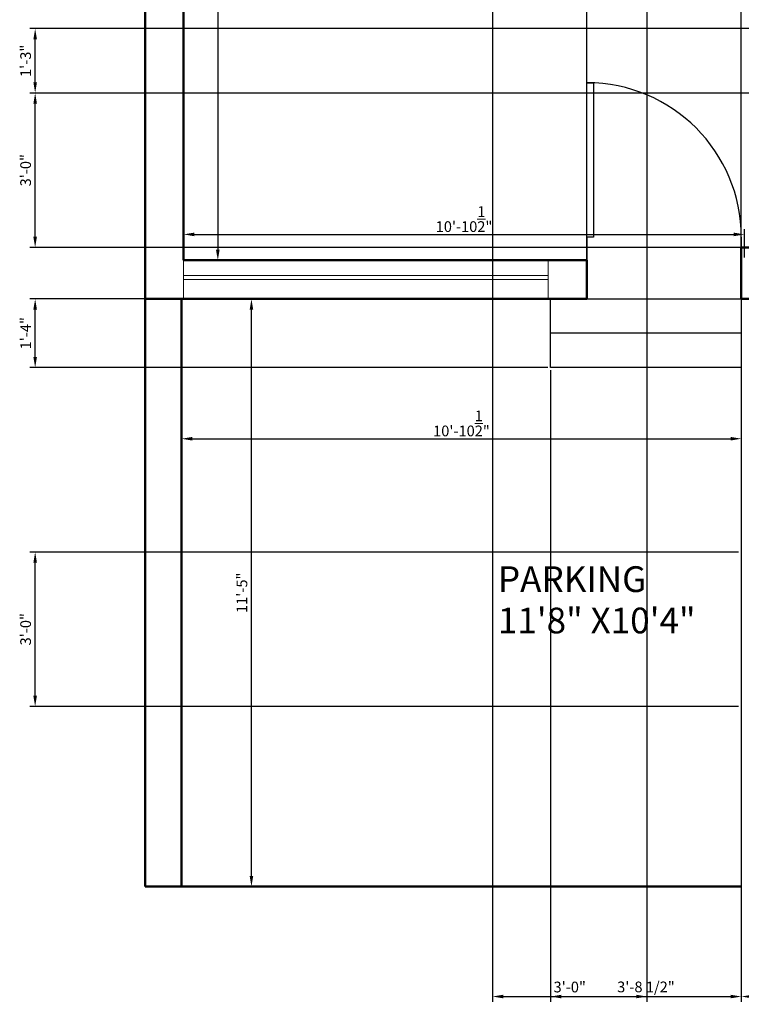
# Model space of a CAD drawing. Units: inches. Extents: x 2385 to 2740, y 1752 to 2305.
# Tile 1 of 15: x 2385 to 2553, y 1752 to 1981. Entities that reach past the tile are written whole.
import ezdxf

# ---------------------------------------------------------------- set-up
doc = ezdxf.new("R2010")
doc.units = ezdxf.units.IN
for name, color, linetype, lineweight in [('A-ANNO-DIMS', 2, 'Continuous', 18), ('A-AREA-IDEN', 7, 'Continuous', 25), ('A-DOOR', 4, 'Continuous', 25), ('A-FLOR-STRS', 7, 'Continuous', 25), ('A-GLAZ', 4, 'Continuous', 18), ('A-WALL', 7, 'Continuous', 50)]:
    doc.layers.add(name, color=color, linetype=linetype, lineweight=lineweight)
doc.styles.get("Standard").update_dxf_attribs({"font": 'arial.ttf'})
doc.dimstyles.new('Copy of ISO-25', dxfattribs={"dimtxt": 2.5, "dimasz": 2.5, "dimexe": 1.25, "dimexo": 0.625, "dimtad": 1, "dimdec": 1, "dimlunit": 4, "dimtxsty": 'Standard', "dimcen": 2.5, "dimadec": 0, "dimazin": 0, "dimtfac": 1, "dimtdec": 1, "dimtmove": 0, "dimatfit": 3, "dimfxl": 1, "dimarcsym": 0})

# ---------------------------------------------------------------- blocks, each defined once
blk = doc.blocks.new('*D12')
at = {"layer": 'A-ANNO-DIMS', "color": 0, "lineweight": -2, "transparency": 16777216}
for p, q in [((2423.87, 2140.97), (2432.46, 2140.97)), ((2431.21, 2138.47), (2431.21, 1927.47)), ((2423.87, 1924.97), (2432.46, 1924.97))]:
    blk.add_line(p, q, dxfattribs=at)
at = {"layer": 'A-ANNO-DIMS', "color": 0, "transparency": 16777216}
for points in [[(2430.79, 2138.47), (2431.63, 2138.47), (2431.21, 2140.97)], [(2430.79, 1927.47), (2431.63, 1927.47), (2431.21, 1924.97)]]:
    blk.add_solid(points, dxfattribs=at)
at = {"layer": 'Defpoints', "color": 0, "transparency": 16777216}
for p in [(2423.25, 2140.97), (2423.25, 1924.97), (2431.21, 1924.97)]:
    blk.add_point(p, dxfattribs=at)
at = {"layer": 'A-ANNO-DIMS', "color": 0, "transparency": 16777216, "insert": (2429.31, 2032.97), "char_height": 2.5, "attachment_point": 5, "rotation": 90}
blk.add_mtext("18'", dxfattribs=at)
blk = doc.blocks.new('*D13')
at = {"layer": 'A-ANNO-DIMS', "color": 0, "lineweight": -2, "transparency": 16777216}
for p, q in [((2423.25, 1925.59), (2423.25, 1932.26)), ((2425.75, 1931.01), (2551.46, 1931.01)), ((2553.96, 1925.59), (2553.96, 1932.26))]:
    blk.add_line(p, q, dxfattribs=at)
at = {"layer": 'A-ANNO-DIMS', "color": 0, "transparency": 16777216}
for points in [[(2425.75, 1931.43), (2425.75, 1930.59), (2423.25, 1931.01)], [(2551.46, 1931.43), (2551.46, 1930.59), (2553.96, 1931.01)]]:
    blk.add_solid(points, dxfattribs=at)
at = {"layer": 'Defpoints', "color": 0, "transparency": 16777216}
for p in [(2553.96, 1931.01), (2423.25, 1924.97), (2553.96, 1924.97)]:
    blk.add_point(p, dxfattribs=at)
at = {"layer": 'A-ANNO-DIMS', "color": 0, "transparency": 16777216, "insert": (2488.61, 1934.58), "char_height": 2.5, "attachment_point": 5}
blk.add_mtext('10\'-10{\\H1x;\\S1/2;}"', dxfattribs=at)
blk = doc.blocks.new('*D20')
at = {"layer": 'A-ANNO-DIMS', "color": 0, "lineweight": -2, "transparency": 16777216}
for p, q in [((2423.4, 1915.97), (2440.3, 1915.97)), ((2439.05, 1781.47), (2439.05, 1913.47)), ((2423.4, 1778.97), (2440.3, 1778.97))]:
    blk.add_line(p, q, dxfattribs=at)
at = {"layer": 'A-ANNO-DIMS', "color": 0, "transparency": 16777216}
for points in [[(2438.64, 1913.47), (2439.47, 1913.47), (2439.05, 1915.97)], [(2438.64, 1781.47), (2439.47, 1781.47), (2439.05, 1778.97)]]:
    blk.add_solid(points, dxfattribs=at)
at = {"layer": 'Defpoints', "color": 0, "transparency": 16777216}
for p in [(2422.77, 1915.97), (2439.05, 1915.97), (2422.77, 1778.97)]:
    blk.add_point(p, dxfattribs=at)
at = {"layer": 'A-ANNO-DIMS', "color": 0, "transparency": 16777216, "insert": (2437.15, 1847.47), "char_height": 2.5, "attachment_point": 5, "rotation": 90}
blk.add_mtext('11\'-5"', dxfattribs=at)
blk = doc.blocks.new('*D21')
at = {"layer": 'A-ANNO-DIMS', "color": 0, "lineweight": -2, "transparency": 16777216}
for p, q in [((2422.77, 1915.34), (2422.77, 1882.13)), ((2553.25, 1915.34), (2553.25, 1882.13)), ((2425.27, 1883.38), (2550.75, 1883.38))]:
    blk.add_line(p, q, dxfattribs=at)
at = {"layer": 'A-ANNO-DIMS', "color": 0, "transparency": 16777216}
for points in [[(2425.27, 1883.8), (2425.27, 1882.96), (2422.77, 1883.38)], [(2550.75, 1883.8), (2550.75, 1882.96), (2553.25, 1883.38)]]:
    blk.add_solid(points, dxfattribs=at)
at = {"layer": 'Defpoints', "color": 0, "transparency": 16777216}
for p in [(2422.77, 1915.97), (2553.25, 1915.97), (2553.25, 1883.38)]:
    blk.add_point(p, dxfattribs=at)
at = {"layer": 'A-ANNO-DIMS', "color": 0, "transparency": 16777216, "insert": (2488.01, 1886.95), "char_height": 2.5, "attachment_point": 5}
blk.add_mtext('10\'-10{\\H1x;\\S1/2;}"', dxfattribs=at)
blk = doc.blocks.new('*U23')
for p, q in [((0, 0), (0, -6)), ((40, 0), (40, -6))]:
    blk.add_line(p, q)
blk.add_lwpolyline([(0, 0), (0, 40), (1.75, 40), (1.75, 0)], close=True)
blk.add_arc((0, 0), 40, 0, 90)
blk = doc.blocks.new('*D34')
at = {"layer": 'A-ANNO-DIMS', "color": 0, "lineweight": -2, "transparency": 16777216}
for p, q in [((2553.25, 1820.34), (2553.25, 1752.1)), ((2651.25, 1820.34), (2651.25, 1752.1)), ((2555.75, 1753.35), (2648.75, 1753.35))]:
    blk.add_line(p, q, dxfattribs=at)
at = {"layer": 'A-ANNO-DIMS', "color": 0, "transparency": 16777216}
for points in [[(2555.75, 1753.77), (2555.75, 1752.94), (2553.25, 1753.35)], [(2648.75, 1753.77), (2648.75, 1752.94), (2651.25, 1753.35)]]:
    blk.add_solid(points, dxfattribs=at)
at = {"layer": 'Defpoints', "color": 0, "transparency": 16777216}
for p in [(2553.25, 1820.97), (2651.25, 1820.97), (2651.25, 1753.35)]:
    blk.add_point(p, dxfattribs=at)
at = {"layer": 'A-ANNO-DIMS', "color": 0, "transparency": 16777216, "insert": (2602.25, 1755.25), "char_height": 2.5, "attachment_point": 5}
blk.add_mtext('8\'-2"', dxfattribs=at)
blk = doc.blocks.new('*D35')
at = {"layer": 'A-ANNO-DIMS', "color": 0, "lineweight": -2, "transparency": 16777216}
for p, q in [((2552.62, 1856.97), (2387.38, 1856.97)), ((2388.63, 1823.47), (2388.63, 1854.47)), ((2552.62, 1820.97), (2387.38, 1820.97))]:
    blk.add_line(p, q, dxfattribs=at)
at = {"layer": 'A-ANNO-DIMS', "color": 0, "transparency": 16777216}
for points in [[(2388.21, 1854.47), (2389.05, 1854.47), (2388.63, 1856.97)], [(2388.21, 1823.47), (2389.05, 1823.47), (2388.63, 1820.97)]]:
    blk.add_solid(points, dxfattribs=at)
at = {"layer": 'Defpoints', "color": 0, "transparency": 16777216}
for p in [(2388.63, 1856.97), (2553.25, 1856.97), (2553.25, 1820.97)]:
    blk.add_point(p, dxfattribs=at)
at = {"layer": 'A-ANNO-DIMS', "color": 0, "transparency": 16777216, "insert": (2386.73, 1838.97), "char_height": 2.5, "attachment_point": 5, "rotation": 90}
blk.add_mtext('3\'-0"', dxfattribs=at)
blk = doc.blocks.new('*D37')
at = {"layer": 'A-ANNO-DIMS', "color": 0, "lineweight": -2, "transparency": 16777216}
for p, q in [((2495.25, 2140.34), (2495.25, 1752.1)), ((2531.25, 2140.34), (2531.25, 1752.1)), ((2497.75, 1753.35), (2528.75, 1753.35))]:
    blk.add_line(p, q, dxfattribs=at)
at = {"layer": 'A-ANNO-DIMS', "color": 0, "transparency": 16777216}
for points in [[(2497.75, 1753.77), (2497.75, 1752.94), (2495.25, 1753.35)], [(2528.75, 1753.77), (2528.75, 1752.94), (2531.25, 1753.35)]]:
    blk.add_solid(points, dxfattribs=at)
at = {"layer": 'Defpoints', "color": 0, "transparency": 16777216}
for p in [(2495.25, 2140.97), (2531.25, 2140.97), (2531.25, 1753.35)]:
    blk.add_point(p, dxfattribs=at)
at = {"layer": 'A-ANNO-DIMS', "color": 0, "transparency": 16777216, "insert": (2513.25, 1755.25), "char_height": 2.5, "attachment_point": 5}
blk.add_mtext('3\'-0"', dxfattribs=at)
blk = doc.blocks.new('*D41')
at = {"layer": 'A-ANNO-DIMS', "color": 0, "lineweight": -2, "transparency": 16777216}
for p, q in [((2558.62, 1978.97), (2387.38, 1978.97)), ((2388.63, 1966.47), (2388.63, 1976.47)), ((2558.62, 1963.97), (2387.38, 1963.97))]:
    blk.add_line(p, q, dxfattribs=at)
at = {"layer": 'A-ANNO-DIMS', "color": 0, "transparency": 16777216}
for points in [[(2388.21, 1976.47), (2389.05, 1976.47), (2388.63, 1978.97)], [(2388.21, 1966.47), (2389.05, 1966.47), (2388.63, 1963.97)]]:
    blk.add_solid(points, dxfattribs=at)
at = {"layer": 'Defpoints', "color": 0, "transparency": 16777216}
for p in [(2388.63, 1978.97), (2559.25, 1978.97), (2559.25, 1963.97)]:
    blk.add_point(p, dxfattribs=at)
at = {"layer": 'A-ANNO-DIMS', "color": 0, "transparency": 16777216, "insert": (2386.73, 1971.47), "char_height": 2.5, "attachment_point": 5, "rotation": 90}
blk.add_mtext('1\'-3"', dxfattribs=at)
blk = doc.blocks.new('*D42')
at = {"layer": 'A-ANNO-DIMS', "color": 0, "lineweight": -2, "transparency": 16777216}
for p, q in [((2558.62, 1963.97), (2387.38, 1963.97)), ((2388.63, 1930.47), (2388.63, 1961.47)), ((2558.62, 1927.97), (2387.38, 1927.97))]:
    blk.add_line(p, q, dxfattribs=at)
at = {"layer": 'A-ANNO-DIMS', "color": 0, "transparency": 16777216}
for points in [[(2388.21, 1961.47), (2389.05, 1961.47), (2388.63, 1963.97)], [(2388.21, 1930.47), (2389.05, 1930.47), (2388.63, 1927.97)]]:
    blk.add_solid(points, dxfattribs=at)
at = {"layer": 'Defpoints', "color": 0, "transparency": 16777216}
for p in [(2388.63, 1963.97), (2559.25, 1963.97), (2559.25, 1927.97)]:
    blk.add_point(p, dxfattribs=at)
at = {"layer": 'A-ANNO-DIMS', "color": 0, "transparency": 16777216, "insert": (2386.73, 1945.97), "char_height": 2.5, "attachment_point": 5, "rotation": 90}
blk.add_mtext('3\'-0"', dxfattribs=at)
blk = doc.blocks.new('*D46')
at = {"layer": 'A-ANNO-DIMS', "color": 0, "lineweight": -2, "transparency": 16777216}
for p, q in [((2508.79, 1899.34), (2508.79, 1752.1)), ((2553.25, 1899.34), (2553.25, 1752.1)), ((2511.29, 1753.35), (2550.75, 1753.35))]:
    blk.add_line(p, q, dxfattribs=at)
at = {"layer": 'A-ANNO-DIMS', "color": 0, "transparency": 16777216}
for points in [[(2511.29, 1753.77), (2511.29, 1752.94), (2508.79, 1753.35)], [(2550.75, 1753.77), (2550.75, 1752.94), (2553.25, 1753.35)]]:
    blk.add_solid(points, dxfattribs=at)
at = {"layer": 'Defpoints', "color": 0, "transparency": 16777216}
for p in [(2508.79, 1899.97), (2553.25, 1899.97), (2553.25, 1753.35)]:
    blk.add_point(p, dxfattribs=at)
at = {"layer": 'A-ANNO-DIMS', "color": 0, "transparency": 16777216, "insert": (2531.02, 1755.27), "char_height": 2.5, "attachment_point": 5}
blk.add_mtext('3\'-8 1/2"', dxfattribs=at)
blk = doc.blocks.new('*D47')
at = {"layer": 'A-ANNO-DIMS', "color": 0, "lineweight": -2, "transparency": 16777216}
for p, q in [((2508.17, 1915.97), (2387.38, 1915.97)), ((2388.63, 1902.47), (2388.63, 1913.47)), ((2508.17, 1899.97), (2387.38, 1899.97))]:
    blk.add_line(p, q, dxfattribs=at)
at = {"layer": 'A-ANNO-DIMS', "color": 0, "transparency": 16777216}
for points in [[(2388.21, 1913.47), (2389.05, 1913.47), (2388.63, 1915.97)], [(2388.21, 1902.47), (2389.05, 1902.47), (2388.63, 1899.97)]]:
    blk.add_solid(points, dxfattribs=at)
at = {"layer": 'Defpoints', "color": 0, "transparency": 16777216}
for p in [(2388.63, 1915.97), (2508.79, 1915.97), (2508.79, 1899.97)]:
    blk.add_point(p, dxfattribs=at)
at = {"layer": 'A-ANNO-DIMS', "color": 0, "transparency": 16777216, "insert": (2386.75, 1907.97), "char_height": 2.5, "attachment_point": 5, "rotation": 90}
blk.add_mtext('1\'-4"', dxfattribs=at)
blk = doc.blocks.new('*D48')
at = {"layer": 'A-ANNO-DIMS', "color": 0, "lineweight": -2, "transparency": 16777216}
for p, q in [((2517.25, 1916.59), (2517.25, 2302.84)), ((2553.25, 1916.59), (2553.25, 2302.84)), ((2519.75, 2301.59), (2550.75, 2301.59))]:
    blk.add_line(p, q, dxfattribs=at)
at = {"layer": 'A-ANNO-DIMS', "color": 0, "transparency": 16777216}
for points in [[(2519.75, 2302), (2519.75, 2301.17), (2517.25, 2301.59)], [(2550.75, 2302), (2550.75, 2301.17), (2553.25, 2301.59)]]:
    blk.add_solid(points, dxfattribs=at)
at = {"layer": 'Defpoints', "color": 0, "transparency": 16777216}
for p in [(2553.25, 2301.59), (2517.25, 1915.97), (2553.25, 1915.97)]:
    blk.add_point(p, dxfattribs=at)
at = {"layer": 'A-ANNO-DIMS', "color": 0, "transparency": 16777216, "insert": (2535.25, 2303.49), "char_height": 2.5, "attachment_point": 5}
blk.add_mtext('3\'-0"', dxfattribs=at)

msp = doc.modelspace()

# ---------------------------------------------------------------- linework, layer by layer
at = {"layer": 'A-FLOR-STRS'}
for p, q in [((2508.79, 1907.97), (2508.79, 1915.97)), ((2517.25, 1915.97), (2553.25, 1915.97)), ((2553.25, 1915.97), (2553.25, 1907.97)), ((2553.25, 1907.97), (2508.79, 1907.97)), ((2508.79, 1899.97), (2508.79, 1907.97)), ((2553.25, 1899.97), (2508.79, 1899.97))]:
    msp.add_line(p, q, dxfattribs=at)
at = {"layer": 'A-GLAZ'}
for p, q in [((2423.25, 1924.97), (2423.25, 1915.97)), ((2508.21, 1924.97), (2508.21, 1915.97)), ((2423.25, 1921.47), (2508.21, 1921.47)), ((2423.25, 1920.47), (2508.21, 1920.47))]:
    msp.add_line(p, q, dxfattribs=at)
at = {"layer": 'A-WALL'}
for p, q in [((2414.25, 1924.97), (2414.25, 2266.97)), ((2423.25, 2140.97), (2423.25, 1924.97)), ((2423.25, 2140.97), (2423.25, 1924.97)), ((2553.25, 1915.96), (2553.25, 1927.97)), ((2553.25, 1915.97), (2553.25, 1927.97)), ((2553.25, 1927.97), (2559.25, 1927.97)), ((2414.25, 1924.97), (2414.25, 1915.97)), ((2423.25, 1924.97), (2517.25, 1924.97)), ((2423.25, 1924.97), (2434.04, 1924.97)), ((2517.25, 1924.97), (2508.21, 1924.97)), ((2517.25, 1915.97), (2517.25, 1924.97)), ((2414.25, 1915.97), (2517.25, 1915.97)), ((2414.25, 1778.97), (2414.25, 1915.97)), ((2414.25, 1915.97), (2422.77, 1915.97)), ((2422.77, 1915.97), (2422.77, 1778.97)), ((2553.25, 1915.97), (2559.25, 1915.97)), ((2553.25, 1778.97), (2414.25, 1778.97))]:
    msp.add_line(p, q, dxfattribs=at)

# ---------------------------------------------------------------- block references
at = {"layer": 'A-DOOR', "xscale": 0.8997681569497455, "yscale": 0.8997681569497455, "zscale": 0.8997681569497455}
msp.add_blockref('*U23', (2517.25, 1930.37), dxfattribs=at)

# ---------------------------------------------------------------- texts
at = {"layer": 'A-AREA-IDEN'}
for s, p in [('PARKING', (2496.5, 1847.65)), ('11\'8" X10\'4"', (2496.5, 1838.01))]:
    msp.add_text(s, height=6, dxfattribs=at).set_placement(p)

# ---------------------------------------------------------------- dimensions: what is measured, and where the dimension line sits
at = {"layer": 'A-ANNO-DIMS'}
for base, p1, p2, override, picture, middle in [((2553.25, 2301.59), (2517.25, 1915.97), (2553.25, 1915.97), {"dimdec": 1, "dimlfac": 1, "dimrnd": 0, "dimzin": 1, "dimdsep": 46, "dimlunit": 4, "dimfrac": 2}, '*D48', (2535.25, 2303.49)), ((2531.25, 1753.35), (2495.25, 2140.97), (2531.25, 2140.97), {"dimdec": 1, "dimlfac": 1, "dimrnd": 0, "dimzin": 1, "dimdsep": 46, "dimlunit": 4, "dimfrac": 2}, '*D37', (2513.25, 1755.25)), ((2553.96, 1931.01), (2423.25, 1924.97), (2553.96, 1924.97), {"dimclrd": 0, "dimclre": 0, "dimclrt": 0}, '*D13', (2488.61, 1934.58)), ((2553.25, 1883.38), (2422.77, 1915.97), (2553.25, 1915.97), {"dimclrd": 0, "dimclre": 0, "dimclrt": 0}, '*D21', (2488.01, 1886.95)), ((2553.25, 1753.35), (2508.79, 1899.97), (2553.25, 1899.97), {"dimdec": 1, "dimlfac": 1, "dimrnd": 0, "dimzin": 1, "dimdsep": 46, "dimlunit": 4, "dimfrac": 2}, '*D46', (2531.02, 1755.27)), ((2651.25, 1753.35), (2553.25, 1820.97), (2651.25, 1820.97), {"dimdec": 1, "dimlfac": 1, "dimrnd": 0, "dimzin": 1, "dimdsep": 46, "dimlunit": 4, "dimfrac": 2}, '*D34', (2602.25, 1755.25))]:
    dim = msp.add_linear_dim(base=base, p1=p1, p2=p2, dimstyle='Copy of ISO-25', override=override, dxfattribs=at)
    dim.commit()
    dim.dimension.update_dxf_attribs({"geometry": picture, "text_midpoint": middle})
for base, p1, p2, override, picture, middle in [((2431.21, 1924.97), (2423.25, 2140.97), (2423.25, 1924.97), {"dimclrd": 0, "dimclre": 0, "dimclrt": 0}, '*D12', (2429.31, 2032.97)), ((2388.63, 1978.97), (2559.25, 1963.97), (2559.25, 1978.97), {"dimdec": 1, "dimlfac": 1, "dimrnd": 0, "dimzin": 1, "dimdsep": 46, "dimlunit": 4, "dimfrac": 2}, '*D41', (2386.73, 1971.47)), ((2388.63, 1963.97), (2559.25, 1927.97), (2559.25, 1963.97), {"dimdec": 1, "dimlfac": 1, "dimrnd": 0, "dimzin": 1, "dimdsep": 46, "dimlunit": 4, "dimfrac": 2}, '*D42', (2386.73, 1945.97)), ((2388.63, 1915.97), (2508.79, 1899.97), (2508.79, 1915.97), {"dimdec": 1, "dimlfac": 1, "dimrnd": 0, "dimzin": 1, "dimdsep": 46, "dimlunit": 4, "dimfrac": 2}, '*D47', (2386.75, 1907.97)), ((2439.05, 1915.97), (2422.77, 1778.97), (2422.77, 1915.97), {"dimclrd": 0, "dimclre": 0, "dimclrt": 0}, '*D20', (2437.15, 1847.47)), ((2388.63, 1856.97), (2553.25, 1820.97), (2553.25, 1856.97), {"dimdec": 1, "dimlfac": 1, "dimrnd": 0, "dimzin": 1, "dimdsep": 46, "dimlunit": 4, "dimfrac": 2}, '*D35', (2386.73, 1838.97))]:
    dim = msp.add_linear_dim(base=base, p1=p1, p2=p2, angle=90, dimstyle='Copy of ISO-25', override=override, dxfattribs=at)
    dim.commit()
    dim.dimension.update_dxf_attribs({"geometry": picture, "text_midpoint": middle})

doc.saveas('drawing.dxf')
